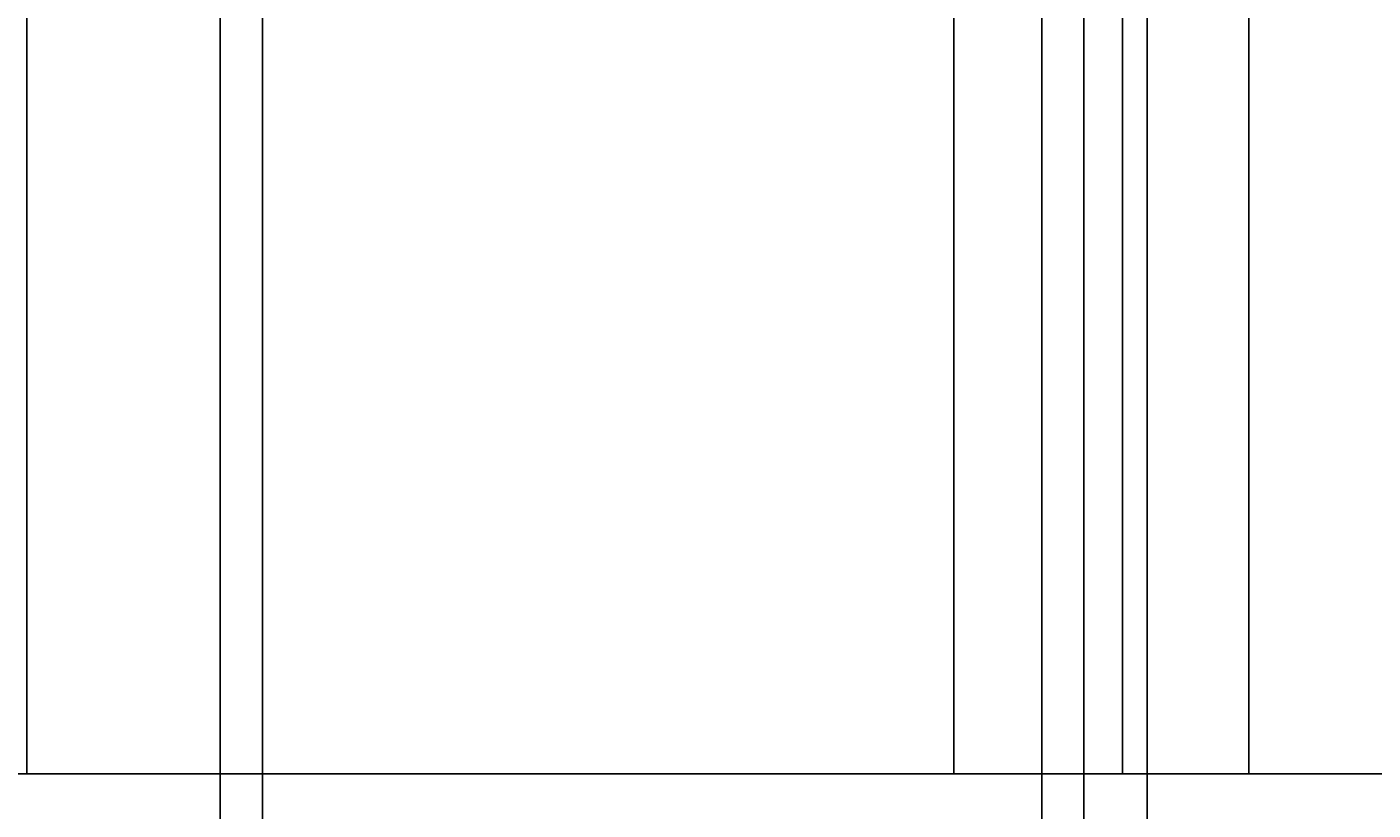
# Model space of a CAD drawing. Units: inches. Extents: x -6 to 289, y -8 to 323.
# Tile 22 of 107: x 142 to 174, y 50 to 69. Entities that reach past the tile are written whole.
import ezdxf

# ---------------------------------------------------------------- set-up
doc = ezdxf.new("R2010")
doc.units = ezdxf.units.IN
doc.header["$MEASUREMENT"] = 0
doc.layers.add('A-ANNO-DIMS', color=2, linetype='Continuous', lineweight=18)
doc.layers.add('A-DOOR', color=3, linetype='Continuous', lineweight=25)
doc.styles.get("Standard").update_dxf_attribs({"font": 'arial.ttf'})
doc.dimstyles.get("Standard").update_dxf_attribs({"dimtxt": 0.18, "dimasz": 0.18, "dimexe": 0.18, "dimexo": 0.0625, "dimgap": 0.09, "dimtad": 0, "dimtih": 1, "dimtoh": 1, "dimdec": 4, "dimzin": 0, "dimdsep": 46, "dimtxsty": 'Standard', "dimcen": 0.09, "dimadec": 0, "dimazin": 0, "dimtfac": 1, "dimtdec": 4, "dimtofl": 0, "dimtmove": 0, "dimatfit": 3, "dimfxl": 1, "dimtolj": 1, "dimtzin": 0, "dimarcsym": 0})

# ---------------------------------------------------------------- blocks, each defined once
blk = doc.blocks.new('*D16')
at = {"layer": 'A-ANNO-DIMS', "color": 0, "lineweight": -2, "transparency": 16777216}
for p, q in [((9.943, 68.37), (9.943, -8.391)), ((272.973, 68.37), (272.973, -8.391)), ((10.123, -8.211), (140.993, -8.211)), ((272.793, -8.211), (141.923, -8.211))]:
    blk.add_line(p, q, dxfattribs=at)
at = {"layer": 'A-ANNO-DIMS', "color": 0, "transparency": 16777216}
for points in [[(10.123, -8.181), (10.123, -8.241), (9.943, -8.211)], [(272.793, -8.181), (272.793, -8.241), (272.973, -8.211)]]:
    blk.add_solid(points, dxfattribs=at)
at = {"layer": 'Defpoints', "color": 0, "transparency": 16777216}
for p in [(9.943, 68.432), (272.973, 68.432), (272.973, -8.211)]:
    blk.add_point(p, dxfattribs=at)
at = {"layer": 'A-ANNO-DIMS', "color": 0, "transparency": 16777216, "insert": (141.458, -8.211), "char_height": 0.18, "attachment_point": 5}
blk.add_mtext('\\A1;263.03', dxfattribs=at)
blk = doc.blocks.new('*D30')
at = {"layer": 'A-ANNO-DIMS', "color": 0, "lineweight": -2, "transparency": 16777216}
for p, q in [((129.383, 181.092), (129.383, -8.391)), ((146.883, 181.092), (146.883, -8.391)), ((129.563, -8.211), (137.817, -8.211)), ((146.703, -8.211), (138.449, -8.211))]:
    blk.add_line(p, q, dxfattribs=at)
at = {"layer": 'A-ANNO-DIMS', "color": 0, "transparency": 16777216}
for points in [[(129.563, -8.181), (129.563, -8.241), (129.383, -8.211)], [(146.703, -8.181), (146.703, -8.241), (146.883, -8.211)]]:
    blk.add_solid(points, dxfattribs=at)
at = {"layer": 'Defpoints', "color": 0, "transparency": 16777216}
for p in [(129.383, 181.154), (146.883, 181.154), (146.883, -8.211)]:
    blk.add_point(p, dxfattribs=at)
at = {"layer": 'A-ANNO-DIMS', "color": 0, "transparency": 16777216, "insert": (138.133, -8.211), "char_height": 0.18, "attachment_point": 5}
blk.add_mtext('\\A1;17.5', dxfattribs=at)
blk = doc.blocks.new('*D31')
at = {"layer": 'A-ANNO-DIMS', "color": 0, "lineweight": -2, "transparency": 16777216}
for p, q in [((146.883, 181.092), (146.883, -8.391)), ((147.883, 181.092), (147.883, -8.391)), ((147.063, -8.211), (147.26, -8.211)), ((147.703, -8.211), (147.507, -8.211))]:
    blk.add_line(p, q, dxfattribs=at)
at = {"layer": 'A-ANNO-DIMS', "color": 0, "transparency": 16777216}
for points in [[(147.063, -8.181), (147.063, -8.241), (146.883, -8.211)], [(147.703, -8.181), (147.703, -8.241), (147.883, -8.211)]]:
    blk.add_solid(points, dxfattribs=at)
at = {"layer": 'Defpoints', "color": 0, "transparency": 16777216}
for p in [(146.883, 181.154), (147.883, 181.154), (147.883, -8.211)]:
    blk.add_point(p, dxfattribs=at)
at = {"layer": 'A-ANNO-DIMS', "color": 0, "transparency": 16777216, "insert": (147.383, -8.211), "char_height": 0.18, "attachment_point": 5}
blk.add_mtext('\\A1;1', dxfattribs=at)
blk = doc.blocks.new('*D32')
at = {"layer": 'A-ANNO-DIMS', "color": 0, "lineweight": -2, "transparency": 16777216}
for p, q in [((147.883, 181.092), (147.883, -8.391)), ((166.383, 181.092), (166.383, -8.391)), ((148.063, -8.211), (156.817, -8.211)), ((166.203, -8.211), (157.449, -8.211))]:
    blk.add_line(p, q, dxfattribs=at)
at = {"layer": 'A-ANNO-DIMS', "color": 0, "transparency": 16777216}
for points in [[(148.063, -8.181), (148.063, -8.241), (147.883, -8.211)], [(166.203, -8.181), (166.203, -8.241), (166.383, -8.211)]]:
    blk.add_solid(points, dxfattribs=at)
at = {"layer": 'Defpoints', "color": 0, "transparency": 16777216}
for p in [(147.883, 181.154), (166.383, 181.154), (166.383, -8.211)]:
    blk.add_point(p, dxfattribs=at)
at = {"layer": 'A-ANNO-DIMS', "color": 0, "transparency": 16777216, "insert": (157.133, -8.211), "char_height": 0.18, "attachment_point": 5}
blk.add_mtext('\\A1;18.5', dxfattribs=at)
blk = doc.blocks.new('*D33')
at = {"layer": 'A-ANNO-DIMS', "color": 0, "lineweight": -2, "transparency": 16777216}
for p, q in [((166.383, 181.092), (166.383, -8.391)), ((167.383, 180.092), (167.383, -8.391)), ((166.563, -8.211), (166.76, -8.211)), ((167.203, -8.211), (167.007, -8.211))]:
    blk.add_line(p, q, dxfattribs=at)
at = {"layer": 'A-ANNO-DIMS', "color": 0, "transparency": 16777216}
for points in [[(166.563, -8.181), (166.563, -8.241), (166.383, -8.211)], [(167.203, -8.181), (167.203, -8.241), (167.383, -8.211)]]:
    blk.add_solid(points, dxfattribs=at)
at = {"layer": 'Defpoints', "color": 0, "transparency": 16777216}
for p in [(166.383, 181.154), (167.383, 180.154), (167.383, -8.211)]:
    blk.add_point(p, dxfattribs=at)
at = {"layer": 'A-ANNO-DIMS', "color": 0, "transparency": 16777216, "insert": (166.883, -8.211), "char_height": 0.18, "attachment_point": 5}
blk.add_mtext('\\A1;1', dxfattribs=at)
blk = doc.blocks.new('*D34')
at = {"layer": 'A-ANNO-DIMS', "color": 0, "lineweight": -2, "transparency": 16777216}
for p, q in [((167.383, 180.092), (167.383, -8.391)), ((168.883, 178.592), (168.883, -8.391)), ((167.563, -8.211), (167.887, -8.211)), ((168.703, -8.211), (168.38, -8.211))]:
    blk.add_line(p, q, dxfattribs=at)
at = {"layer": 'A-ANNO-DIMS', "color": 0, "transparency": 16777216}
for points in [[(167.563, -8.181), (167.563, -8.241), (167.383, -8.211)], [(168.703, -8.181), (168.703, -8.241), (168.883, -8.211)]]:
    blk.add_solid(points, dxfattribs=at)
at = {"layer": 'Defpoints', "color": 0, "transparency": 16777216}
for p in [(167.383, 180.154), (168.883, 178.654), (168.883, -8.211)]:
    blk.add_point(p, dxfattribs=at)
at = {"layer": 'A-ANNO-DIMS', "color": 0, "transparency": 16777216, "insert": (168.133, -8.211), "char_height": 0.18, "attachment_point": 5}
blk.add_mtext('\\A1;1.5', dxfattribs=at)
blk = doc.blocks.new('*D76')
at = {"layer": 'A-ANNO-DIMS', "color": 0, "lineweight": -2, "transparency": 16777216}
for p, q in [((142.296, 51.148), (142.296, 322.969)), ((142.476, 322.789), (153.076, 322.789)), ((164.116, 322.789), (153.516, 322.789)), ((164.296, 51.148), (164.296, 322.969))]:
    blk.add_line(p, q, dxfattribs=at)
at = {"layer": 'A-ANNO-DIMS', "color": 0, "transparency": 16777216}
for points in [[(142.476, 322.819), (142.476, 322.759), (142.296, 322.789)], [(164.116, 322.819), (164.116, 322.759), (164.296, 322.789)]]:
    blk.add_solid(points, dxfattribs=at)
at = {"layer": 'Defpoints', "color": 0, "transparency": 16777216}
for p in [(164.296, 322.789), (142.296, 51.085), (164.296, 51.085)]:
    blk.add_point(p, dxfattribs=at)
at = {"layer": 'A-ANNO-DIMS', "color": 0, "transparency": 16777216, "insert": (153.296, 322.789), "char_height": 0.18, "attachment_point": 5}
blk.add_mtext('\\A1;22', dxfattribs=at)
blk = doc.blocks.new('*D77')
at = {"layer": 'A-ANNO-DIMS', "color": 0, "lineweight": -2, "transparency": 16777216}
for p, q in [((164.296, 51.148), (164.296, 322.969)), ((164.476, 322.789), (166.144, 322.789)), ((168.116, 322.789), (166.448, 322.789)), ((168.296, 51.148), (168.296, 322.969))]:
    blk.add_line(p, q, dxfattribs=at)
at = {"layer": 'A-ANNO-DIMS', "color": 0, "transparency": 16777216}
for points in [[(164.476, 322.819), (164.476, 322.759), (164.296, 322.789)], [(168.116, 322.819), (168.116, 322.759), (168.296, 322.789)]]:
    blk.add_solid(points, dxfattribs=at)
at = {"layer": 'Defpoints', "color": 0, "transparency": 16777216}
for p in [(168.296, 322.789), (164.296, 51.085), (168.296, 51.085)]:
    blk.add_point(p, dxfattribs=at)
at = {"layer": 'A-ANNO-DIMS', "color": 0, "transparency": 16777216, "insert": (166.296, 322.789), "char_height": 0.18, "attachment_point": 5}
blk.add_mtext('\\A1;4', dxfattribs=at)
blk = doc.blocks.new('*D78')
at = {"layer": 'A-ANNO-DIMS', "color": 0, "lineweight": -2, "transparency": 16777216}
for p, q in [((168.296, 51.148), (168.296, 322.969)), ((168.476, 322.789), (169.647, 322.789)), ((171.116, 322.789), (169.945, 322.789)), ((171.296, 51.148), (171.296, 322.969))]:
    blk.add_line(p, q, dxfattribs=at)
at = {"layer": 'A-ANNO-DIMS', "color": 0, "transparency": 16777216}
for points in [[(168.476, 322.819), (168.476, 322.759), (168.296, 322.789)], [(171.116, 322.819), (171.116, 322.759), (171.296, 322.789)]]:
    blk.add_solid(points, dxfattribs=at)
at = {"layer": 'Defpoints', "color": 0, "transparency": 16777216}
for p in [(171.296, 322.789), (168.296, 51.085), (171.296, 51.085)]:
    blk.add_point(p, dxfattribs=at)
at = {"layer": 'A-ANNO-DIMS', "color": 0, "transparency": 16777216, "insert": (169.796, 322.789), "char_height": 0.18, "attachment_point": 5}
blk.add_mtext('\\A1;3', dxfattribs=at)
blk = doc.blocks.new('*D86')
at = {"layer": 'A-ANNO-DIMS', "color": 0, "lineweight": -2, "transparency": 16777216}
for p, q in [((166.233, 75.971), (-5.737, 75.971)), ((-5.557, 75.791), (-5.557, 63.71)), ((-5.557, 51.265), (-5.557, 63.346)), ((120.945, 51.085), (-5.737, 51.085))]:
    blk.add_line(p, q, dxfattribs=at)
at = {"layer": 'A-ANNO-DIMS', "color": 0, "transparency": 16777216}
for points in [[(-5.587, 75.791), (-5.527, 75.791), (-5.557, 75.971)], [(-5.587, 51.265), (-5.527, 51.265), (-5.557, 51.085)]]:
    blk.add_solid(points, dxfattribs=at)
at = {"layer": 'Defpoints', "color": 0, "transparency": 16777216}
for p in [(-5.557, 75.971), (166.296, 75.971), (121.008, 51.085)]:
    blk.add_point(p, dxfattribs=at)
at = {"layer": 'A-ANNO-DIMS', "color": 0, "transparency": 16777216, "insert": (-5.557, 63.528), "char_height": 0.18, "attachment_point": 5}
blk.add_mtext('\\A1;24.886', dxfattribs=at)

msp = doc.modelspace()

# ---------------------------------------------------------------- linework, layer by layer
at = {"layer": 'A-DOOR'}
for points in [[(135.296, 51.0851), (135.296, 117.9706), (171.296, 117.9706), (171.296, 51.0851)], [(138.296, 51.0851), (138.296, 114.9477), (168.296, 114.9477), (168.296, 51.0851)], [(164.296, 51.0851), (164.296, 108.9477), (142.296, 108.9477), (142.296, 51.0851)]]:
    msp.add_lwpolyline(points, dxfattribs=at)
msp.add_lwpolyline([(121.008, 51.0851), (247.2408, 51.0851), (247.2408, 7.2888), (121.008, 7.2888)], close=True, dxfattribs=at)

# ---------------------------------------------------------------- dimensions: what is measured, and where the dimension line sits
at = {"layer": 'A-ANNO-DIMS'}
for base, p1, p2, override, picture, middle in [((164.296, 322.7888), (142.296, 51.0851), (164.296, 51.0851), {"dimdec": 0, "dimlfac": 1, "dimrnd": 0, "dimzin": 0, "dimdsep": 46, "dimlunit": 2}, '*D76', (153.296, 322.7888)), ((168.296, 322.7888), (164.296, 51.0851), (168.296, 51.0851), {"dimdec": 0, "dimlfac": 1, "dimrnd": 0, "dimzin": 0, "dimdsep": 46, "dimlunit": 2}, '*D77', (166.296, 322.7888)), ((171.296, 322.7888), (168.296, 51.0851), (171.296, 51.0851), {"dimdec": 0, "dimlfac": 1, "dimrnd": 0, "dimzin": 0, "dimdsep": 46, "dimlunit": 2}, '*D78', (169.796, 322.7888)), ((146.8835, -8.2112), (129.3835, 181.154), (146.8835, 181.154), {"dimdec": 1, "dimlfac": 1, "dimrnd": 0, "dimzin": 0, "dimdsep": 46, "dimlunit": 2}, '*D30', (138.1335, -8.2112)), ((147.8835, -8.2112), (146.8835, 181.154), (147.8835, 181.154), {"dimdec": 0, "dimlfac": 1, "dimrnd": 0, "dimzin": 0, "dimdsep": 46, "dimlunit": 2}, '*D31', (147.3835, -8.2112)), ((166.3835, -8.2112), (147.8835, 181.154), (166.3835, 181.154), {"dimdec": 1, "dimlfac": 1, "dimrnd": 0, "dimzin": 0, "dimdsep": 46, "dimlunit": 2}, '*D32', (157.1335, -8.2112)), ((167.3835, -8.2112), (166.3835, 181.154), (167.3835, 180.154), {"dimdec": 0, "dimlfac": 1, "dimrnd": 0, "dimzin": 0, "dimdsep": 46, "dimlunit": 2}, '*D33', (166.8835, -8.2112)), ((168.8835, -8.2112), (167.3835, 180.154), (168.8835, 178.654), {"dimdec": 1, "dimlfac": 1, "dimrnd": 0, "dimzin": 0, "dimdsep": 46, "dimlunit": 2}, '*D34', (168.1335, -8.2112)), ((272.9733, -8.2112), (9.943, 68.4322), (272.9733, 68.4322), {"dimdec": 2, "dimlfac": 1, "dimrnd": 0, "dimzin": 0, "dimdsep": 46, "dimlunit": 2}, '*D16', (141.4581, -8.2112))]:
    dim = msp.add_linear_dim(base=base, p1=p1, p2=p2, dimstyle='Standard', override=override, dxfattribs=at)
    dim.commit()
    dim.dimension.update_dxf_attribs({"geometry": picture, "text_midpoint": middle})
dim = msp.add_linear_dim(base=(-5.557, 75.97064), p1=(121.00798, 51.08513), p2=(166.29599, 75.97064), angle=90, dimstyle='Standard', override={"dimdec": 3, "dimlfac": 1, "dimrnd": 0, "dimzin": 0, "dimdsep": 46, "dimlunit": 2}, dxfattribs=at)
dim.commit()
dim.dimension.update_dxf_attribs({"geometry": '*D86', "text_midpoint": (-5.557, 63.52788)})

doc.saveas('drawing.dxf')
